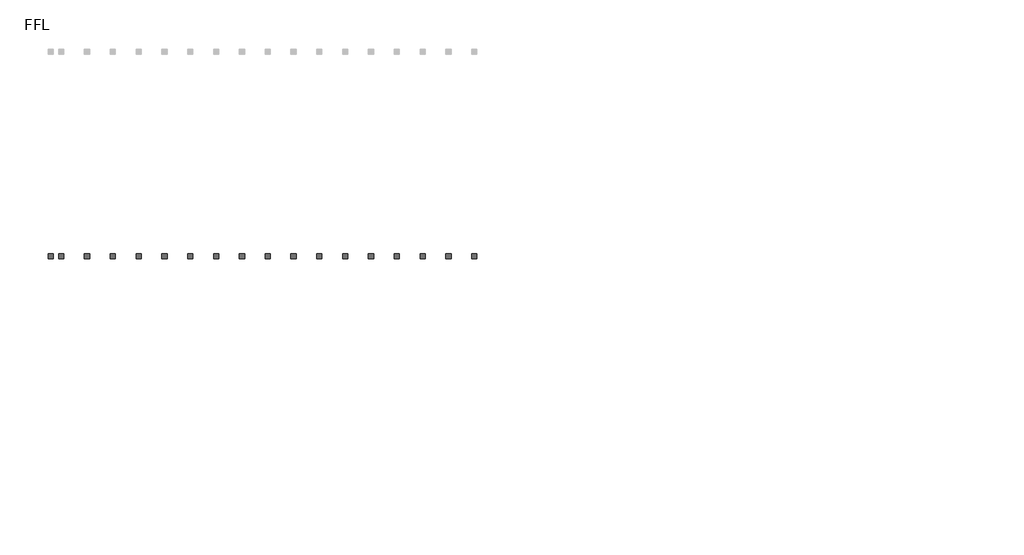
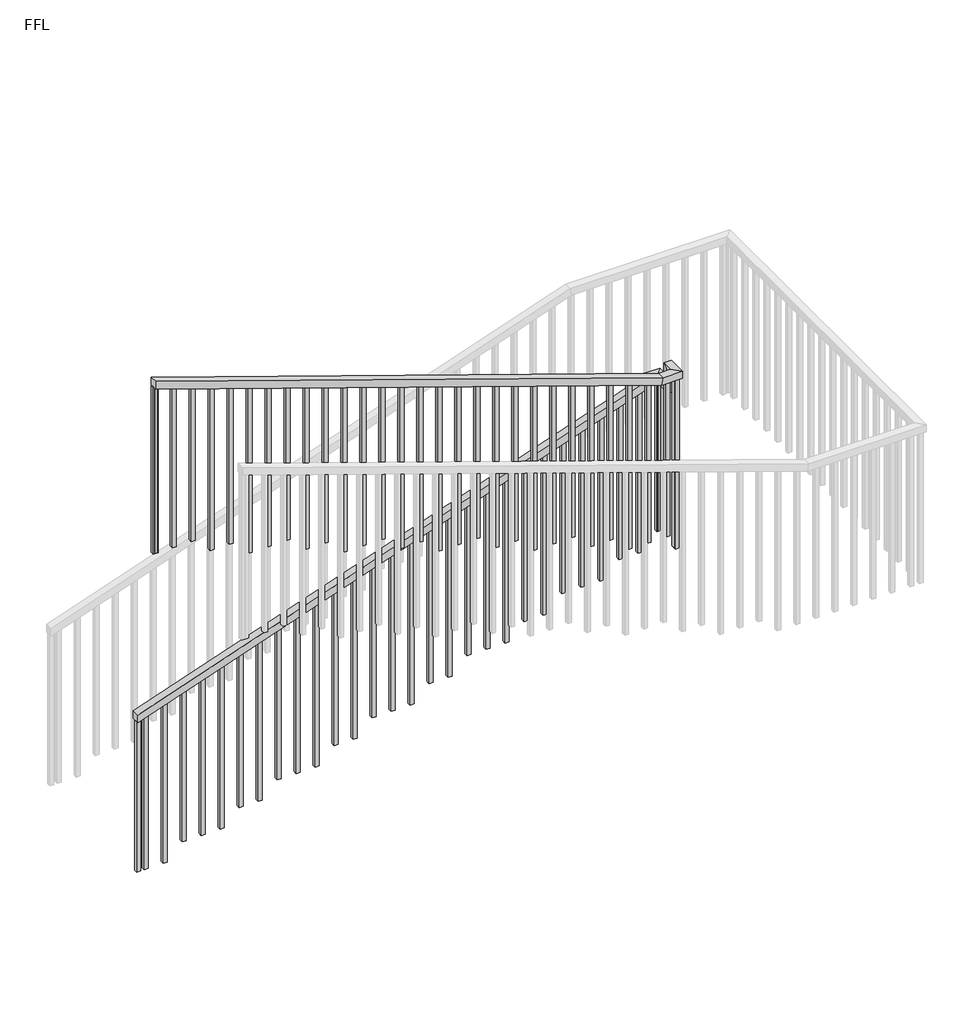
# One storey, part 1 of 2: 1 railing.
"""IFC4 building model written with IfcOpenShell, lengths in millimetres."""

from ifc_helpers import new_model, si_unit, frame, origin, place, context, project, spatial, polyline, outline, extrude, faceted_brep, element, save

model = new_model("IFC4")

# Units and contexts
model_context = context("Model", 3, world=origin())
ifc_project = project(units=[si_unit("LENGTHUNIT", "METRE", prefix="MILLI")], contexts=[model_context])

# Site, building, storey
site = spatial("IfcSite", under=ifc_project)
building = spatial("IfcBuilding", under=site)
storey = spatial("IfcBuildingStorey", under=building, Name="FFL", Elevation=3000.0)

# Railing
placement = place(None, origin())
element("IfcRailing", 1, ObjectType="1100mm", at=placement, inside=storey, context=model_context, shape_type="SolidModel", body=[
    faceted_brep([(-40149.9681829, 16845.7531621, 4656.2088216), (-40149.9681829, 16845.7531621, 4603.3636913), (-40149.9681829, 16795.7531621, 4603.3636913), (-40149.9681829, 16795.7531621, 4656.2088216), (-36808.2681829, 16845.7531621, 5799.4566882), (-36758.2681829, 16845.7531621, 5763.7173404), (-36758.2681829, 16795.7531621, 5763.7173404), (-36808.2681829, 16795.7531621, 5799.4566882), (-36808.2681829, 16845.7531621, 5824.9785156), (-36758.2681829, 16845.7531621, 5774.9785156), (-36758.2681829, 16795.7531621, 5774.9785156), (-36808.2681829, 16795.7531621, 5824.9785156), (-36683.2681829, 16845.7531621, 5824.9785156), (-36683.2681829, 16845.7531621, 5774.9785156), (-36733.2681829, 16795.7531621, 5774.9785156), (-36733.2681829, 16795.7531621, 5824.9785156), (-36683.2681829, 16720.7531621, 5824.9785156), (-36683.2681829, 16720.7531621, 5774.9785156), (-36733.2681829, 16720.7531621, 5774.9785156), (-36733.2681829, 16720.7531621, 5824.9785156), (-36683.2681829, 16717.5531621, 5824.9785156), (-36683.2681829, 16667.5531621, 5774.9785156), (-36733.2681829, 16667.5531621, 5774.9785156), (-36733.2681829, 16717.5531621, 5824.9785156), (-36683.2681829, 16717.5531621, 5956.7521335), (-36683.2681829, 16667.5531621, 5906.7521335), (-36733.2681829, 16667.5531621, 5906.7521335), (-36733.2681829, 16717.5531621, 5956.7521335), (-36683.2681829, 16592.5531621, 5956.7521335), (-36683.2681829, 16592.5531621, 5906.7521335), (-36733.2681829, 16642.5531621, 5906.7521335), (-36733.2681829, 16642.5531621, 5956.7521335), (-36808.2681829, 16592.5531621, 5956.7521335), (-36816.5844651, 16592.5531621, 5906.7521335), (-36816.5844651, 16642.5531621, 5906.7521335), (-36808.2681829, 16642.5531621, 5956.7521335), (-40149.9681829, 16592.5531621, 7100.0), (-40149.9681829, 16642.5531621, 7100.0), (-40149.9681829, 16642.5531621, 7047.1548697), (-40149.9681829, 16592.5531621, 7047.1548697)], [[[0, 1, 2, 3]], [[1, 0, 4, 5]], [[2, 1, 5, 6]], [[3, 2, 6, 7]], [[0, 3, 7, 4]], [[5, 4, 8, 9]], [[6, 5, 9, 10]], [[7, 6, 10, 11]], [[4, 7, 11, 8]], [[9, 8, 12, 13]], [[10, 9, 13, 14]], [[11, 10, 14, 15]], [[8, 11, 15, 12]], [[13, 12, 16, 17]], [[14, 13, 17, 18]], [[15, 14, 18, 19]], [[12, 15, 19, 16]], [[17, 16, 20, 21]], [[18, 17, 21, 22]], [[19, 18, 22, 23]], [[16, 19, 23, 20]], [[21, 20, 24, 25]], [[22, 21, 25, 26]], [[23, 22, 26, 27]], [[20, 23, 27, 24]], [[25, 24, 28, 29]], [[26, 25, 29, 30]], [[27, 26, 30, 31]], [[24, 27, 31, 28]], [[29, 28, 32, 33]], [[30, 29, 33, 34]], [[31, 30, 34, 35]], [[28, 31, 35, 32]], [[36, 37, 38, 39]], [[33, 32, 36, 39]], [[34, 33, 39, 38]], [[35, 34, 38, 37]], [[32, 35, 37, 36]]]),
    extrude(outline(polyline([(5893.7482096, -40133.2681829), (7041.4415384, -40133.2681829), (7049.9944296, -40158.2681829), (5893.7482096, -40158.2681829), (5893.7482096, -40133.2681829)])), frame((0.0, 16605.0531621, 0.0), z_axis=(0.0, 1.0, 0.0), x_axis=(0.0, 0.0, 1.0)), (0.0, 0.0, 1.0), 25.0),
    extrude(outline(polyline([(5893.7482096, -40008.2681829), (6998.6770822, -40008.2681829), (7007.2299734, -40033.2681829), (5893.7482096, -40033.2681829), (5893.7482096, -40008.2681829)])), frame((0.0, 16605.0531621, 0.0), z_axis=(0.0, 1.0, 0.0), x_axis=(0.0, 0.0, 1.0)), (0.0, 0.0, 1.0), 25.0),
    extrude(outline(polyline([(5893.7482096, -39883.2681829), (6955.9126259, -39883.2681829), (6964.4655172, -39908.2681829), (5893.7482096, -39908.2681829), (5893.7482096, -39883.2681829)])), frame((0.0, 16605.0531621, 0.0), z_axis=(0.0, 1.0, 0.0), x_axis=(0.0, 0.0, 1.0)), (0.0, 0.0, 1.0), 25.0),
    extrude(outline(polyline([(5787.4964193, -39758.2681829), (6913.1481697, -39758.2681829), (6921.701061, -39783.2681829), (5787.4964193, -39783.2681829), (5787.4964193, -39758.2681829)])), frame((0.0, 16605.0531621, 0.0), z_axis=(0.0, 1.0, 0.0), x_axis=(0.0, 0.0, 1.0)), (0.0, 0.0, 1.0), 25.0),
    extrude(outline(polyline([(5787.4964193, -39633.2681829), (6870.3837135, -39633.2681829), (6878.9366048, -39658.2681829), (5787.4964193, -39658.2681829), (5787.4964193, -39633.2681829)])), frame((0.0, 16605.0531621, 0.0), z_axis=(0.0, 1.0, 0.0), x_axis=(0.0, 0.0, 1.0)), (0.0, 0.0, 1.0), 25.0),
    extrude(outline(polyline([(5681.2446289, -39508.2681829), (6827.6192573, -39508.2681829), (6836.1721486, -39533.2681829), (5681.2446289, -39533.2681829), (5681.2446289, -39508.2681829)])), frame((0.0, 16605.0531621, 0.0), z_axis=(0.0, 1.0, 0.0), x_axis=(0.0, 0.0, 1.0)), (0.0, 0.0, 1.0), 25.0),
    extrude(outline(polyline([(5681.2446289, -39383.2681829), (6784.8548011, -39383.2681829), (6793.4076923, -39408.2681829), (5681.2446289, -39408.2681829), (5681.2446289, -39383.2681829)])), frame((0.0, 16605.0531621, 0.0), z_axis=(0.0, 1.0, 0.0), x_axis=(0.0, 0.0, 1.0)), (0.0, 0.0, 1.0), 25.0),
    extrude(outline(polyline([(5681.2446289, -39258.2681829), (6742.0903449, -39258.2681829), (6750.6432361, -39283.2681829), (5681.2446289, -39283.2681829), (5681.2446289, -39258.2681829)])), frame((0.0, 16605.0531621, 0.0), z_axis=(0.0, 1.0, 0.0), x_axis=(0.0, 0.0, 1.0)), (0.0, 0.0, 1.0), 25.0),
    extrude(outline(polyline([(5574.9928385, -39133.2681829), (6699.3258887, -39133.2681829), (6707.8787799, -39158.2681829), (5574.9928385, -39158.2681829), (5574.9928385, -39133.2681829)])), frame((0.0, 16605.0531621, 0.0), z_axis=(0.0, 1.0, 0.0), x_axis=(0.0, 0.0, 1.0)), (0.0, 0.0, 1.0), 25.0),
    extrude(outline(polyline([(5574.9928385, -39008.2681829), (6656.5614325, -39008.2681829), (6665.1143237, -39033.2681829), (5574.9928385, -39033.2681829), (5574.9928385, -39008.2681829)])), frame((0.0, 16605.0531621, 0.0), z_axis=(0.0, 1.0, 0.0), x_axis=(0.0, 0.0, 1.0)), (0.0, 0.0, 1.0), 25.0),
    extrude(outline(polyline([(5468.7410482, -38883.2681829), (6613.7969763, -38883.2681829), (6622.3498675, -38908.2681829), (5468.7410482, -38908.2681829), (5468.7410482, -38883.2681829)])), frame((0.0, 16605.0531621, 0.0), z_axis=(0.0, 1.0, 0.0), x_axis=(0.0, 0.0, 1.0)), (0.0, 0.0, 1.0), 25.0),
    extrude(outline(polyline([(5468.7410482, -38758.2681829), (6571.0325201, -38758.2681829), (6579.5854113, -38783.2681829), (5468.7410482, -38783.2681829), (5468.7410482, -38758.2681829)])), frame((0.0, 16605.0531621, 0.0), z_axis=(0.0, 1.0, 0.0), x_axis=(0.0, 0.0, 1.0)), (0.0, 0.0, 1.0), 25.0),
    extrude(outline(polyline([(5468.7410482, -38633.2681829), (6528.2680638, -38633.2681829), (6536.8209551, -38658.2681829), (5468.7410482, -38658.2681829), (5468.7410482, -38633.2681829)])), frame((0.0, 16605.0531621, 0.0), z_axis=(0.0, 1.0, 0.0), x_axis=(0.0, 0.0, 1.0)), (0.0, 0.0, 1.0), 25.0),
    extrude(outline(polyline([(5362.4892578, -38508.2681829), (6485.5036076, -38508.2681829), (6494.0564989, -38533.2681829), (5362.4892578, -38533.2681829), (5362.4892578, -38508.2681829)])), frame((0.0, 16605.0531621, 0.0), z_axis=(0.0, 1.0, 0.0), x_axis=(0.0, 0.0, 1.0)), (0.0, 0.0, 1.0), 25.0),
    extrude(outline(polyline([(5362.4892578, -38383.2681829), (6442.7391514, -38383.2681829), (6451.2920427, -38408.2681829), (5362.4892578, -38408.2681829), (5362.4892578, -38383.2681829)])), frame((0.0, 16605.0531621, 0.0), z_axis=(0.0, 1.0, 0.0), x_axis=(0.0, 0.0, 1.0)), (0.0, 0.0, 1.0), 25.0),
    extrude(outline(polyline([(5256.2374674, -38258.2681829), (6399.9746952, -38258.2681829), (6408.5275865, -38283.2681829), (5256.2374674, -38283.2681829), (5256.2374674, -38258.2681829)])), frame((0.0, 16605.0531621, 0.0), z_axis=(0.0, 1.0, 0.0), x_axis=(0.0, 0.0, 1.0)), (0.0, 0.0, 1.0), 25.0),
    extrude(outline(polyline([(5256.2374674, -38133.2681829), (6357.210239, -38133.2681829), (6365.7631302, -38158.2681829), (5256.2374674, -38158.2681829), (5256.2374674, -38133.2681829)])), frame((0.0, 16605.0531621, 0.0), z_axis=(0.0, 1.0, 0.0), x_axis=(0.0, 0.0, 1.0)), (0.0, 0.0, 1.0), 25.0),
    extrude(outline(polyline([(5256.2374674, -38008.2681829), (6314.4457828, -38008.2681829), (6322.998674, -38033.2681829), (5256.2374674, -38033.2681829), (5256.2374674, -38008.2681829)])), frame((0.0, 16605.0531621, 0.0), z_axis=(0.0, 1.0, 0.0), x_axis=(0.0, 0.0, 1.0)), (0.0, 0.0, 1.0), 25.0),
    extrude(outline(polyline([(5149.9856771, -37883.2681829), (6271.6813266, -37883.2681829), (6280.2342178, -37908.2681829), (5149.9856771, -37908.2681829), (5149.9856771, -37883.2681829)])), frame((0.0, 16605.0531621, 0.0), z_axis=(0.0, 1.0, 0.0), x_axis=(0.0, 0.0, 1.0)), (0.0, 0.0, 1.0), 25.0),
    extrude(outline(polyline([(5149.9856771, -37758.2681829), (6228.9168704, -37758.2681829), (6237.4697616, -37783.2681829), (5149.9856771, -37783.2681829), (5149.9856771, -37758.2681829)])), frame((0.0, 16605.0531621, 0.0), z_axis=(0.0, 1.0, 0.0), x_axis=(0.0, 0.0, 1.0)), (0.0, 0.0, 1.0), 25.0),
    extrude(outline(polyline([(5043.7338867, -37633.2681829), (6186.1524142, -37633.2681829), (6194.7053054, -37658.2681829), (5043.7338867, -37658.2681829), (5043.7338867, -37633.2681829)])), frame((0.0, 16605.0531621, 0.0), z_axis=(0.0, 1.0, 0.0), x_axis=(0.0, 0.0, 1.0)), (0.0, 0.0, 1.0), 25.0),
    extrude(outline(polyline([(5043.7338867, -37508.2681829), (6143.387958, -37508.2681829), (6151.9408492, -37533.2681829), (5043.7338867, -37533.2681829), (5043.7338867, -37508.2681829)])), frame((0.0, 16605.0531621, 0.0), z_axis=(0.0, 1.0, 0.0), x_axis=(0.0, 0.0, 1.0)), (0.0, 0.0, 1.0), 25.0),
    extrude(outline(polyline([(5043.7338867, -37383.2681829), (6100.6235017, -37383.2681829), (6109.176393, -37408.2681829), (5043.7338867, -37408.2681829), (5043.7338867, -37383.2681829)])), frame((0.0, 16605.0531621, 0.0), z_axis=(0.0, 1.0, 0.0), x_axis=(0.0, 0.0, 1.0)), (0.0, 0.0, 1.0), 25.0),
    extrude(outline(polyline([(4937.4820964, -37258.2681829), (6057.8590455, -37258.2681829), (6066.4119368, -37283.2681829), (4937.4820964, -37283.2681829), (4937.4820964, -37258.2681829)])), frame((0.0, 16605.0531621, 0.0), z_axis=(0.0, 1.0, 0.0), x_axis=(0.0, 0.0, 1.0)), (0.0, 0.0, 1.0), 25.0),
    extrude(outline(polyline([(4937.4820964, -37133.2681829), (6015.0945893, -37133.2681829), (6023.6474806, -37158.2681829), (4937.4820964, -37158.2681829), (4937.4820964, -37133.2681829)])), frame((0.0, 16605.0531621, 0.0), z_axis=(0.0, 1.0, 0.0), x_axis=(0.0, 0.0, 1.0)), (0.0, 0.0, 1.0), 25.0),
    extrude(outline(polyline([(4831.230306, -37008.2681829), (5972.3301331, -37008.2681829), (5980.8830244, -37033.2681829), (4831.230306, -37033.2681829), (4831.230306, -37008.2681829)])), frame((0.0, 16605.0531621, 0.0), z_axis=(0.0, 1.0, 0.0), x_axis=(0.0, 0.0, 1.0)), (0.0, 0.0, 1.0), 25.0),
    extrude(outline(polyline([(4831.230306, -36883.2681829), (5929.5656769, -36883.2681829), (5938.1185681, -36908.2681829), (4831.230306, -36908.2681829), (4831.230306, -36883.2681829)])), frame((0.0, 16605.0531621, 0.0), z_axis=(0.0, 1.0, 0.0), x_axis=(0.0, 0.0, 1.0)), (0.0, 0.0, 1.0), 25.0),
    extrude(outline(polyline([(-36758.2681829, 16630.0531621), (-36758.2681829, 16605.0531621), (-36783.2681829, 16605.0531621), (-36783.2681829, 16630.0531621), (-36758.2681829, 16630.0531621)])), frame((0.0, 0.0, 4831.230306), z_axis=(0.0, 0.0, 1.0), x_axis=(1.0, 0.0, 0.0)), (0.0, 0.0, 1.0), 1075.5218275),
    extrude(outline(polyline([(-36720.7681829, 16645.7531621), (-36695.7681829, 16645.7531621), (-36695.7681829, 16620.7531621), (-36720.7681829, 16620.7531621), (-36720.7681829, 16645.7531621)])), frame((0.0, 0.0, 4724.9785156), z_axis=(0.0, 0.0, 1.0), x_axis=(1.0, 0.0, 0.0)), (0.0, 0.0, 1.0), 1181.7736178),
    extrude(outline(polyline([(-36720.7681829, 16770.7531621), (-36695.7681829, 16770.7531621), (-36695.7681829, 16745.7531621), (-36720.7681829, 16745.7531621), (-36720.7681829, 16770.7531621)])), frame((0.0, 0.0, 4724.9785156), z_axis=(0.0, 0.0, 1.0), x_axis=(1.0, 0.0, 0.0)), (0.0, 0.0, 1.0), 1050.0),
    extrude(outline(polyline([(-36724.9681829, 16808.2531621), (-36724.9681829, 16833.2531621), (-36699.9681829, 16833.2531621), (-36699.9681829, 16808.2531621), (-36724.9681829, 16808.2531621)])), frame((0.0, 0.0, 4724.9785156), z_axis=(0.0, 0.0, 1.0), x_axis=(1.0, 0.0, 0.0)), (0.0, 0.0, 1.0), 1050.0),
    extrude(outline(polyline([(5732.3453353, -36849.9681829), (4618.7267253, -36849.9681829), (4618.7267253, -36824.9681829), (5740.8982265, -36824.9681829), (5732.3453353, -36849.9681829)])), frame((0.0, 16808.2531621, 0.0), z_axis=(0.0, 1.0, 0.0), x_axis=(0.0, 0.0, 1.0)), (0.0, 0.0, 1.0), 25.0),
    extrude(outline(polyline([(5689.5808791, -36974.9681829), (4618.7267253, -36974.9681829), (4618.7267253, -36949.9681829), (5698.1337703, -36949.9681829), (5689.5808791, -36974.9681829)])), frame((0.0, 16808.2531621, 0.0), z_axis=(0.0, 1.0, 0.0), x_axis=(0.0, 0.0, 1.0)), (0.0, 0.0, 1.0), 25.0),
    extrude(outline(polyline([(5646.8164229, -37099.9681829), (4512.4749349, -37099.9681829), (4512.4749349, -37074.9681829), (5655.3693141, -37074.9681829), (5646.8164229, -37099.9681829)])), frame((0.0, 16808.2531621, 0.0), z_axis=(0.0, 1.0, 0.0), x_axis=(0.0, 0.0, 1.0)), (0.0, 0.0, 1.0), 25.0),
    extrude(outline(polyline([(5604.0519667, -37224.9681829), (4512.4749349, -37224.9681829), (4512.4749349, -37199.9681829), (5612.6048579, -37199.9681829), (5604.0519667, -37224.9681829)])), frame((0.0, 16808.2531621, 0.0), z_axis=(0.0, 1.0, 0.0), x_axis=(0.0, 0.0, 1.0)), (0.0, 0.0, 1.0), 25.0),
    extrude(outline(polyline([(5561.2875104, -37349.9681829), (4512.4749349, -37349.9681829), (4512.4749349, -37324.9681829), (5569.8404017, -37324.9681829), (5561.2875104, -37349.9681829)])), frame((0.0, 16808.2531621, 0.0), z_axis=(0.0, 1.0, 0.0), x_axis=(0.0, 0.0, 1.0)), (0.0, 0.0, 1.0), 25.0),
    extrude(outline(polyline([(5518.5230542, -37474.9681829), (4406.2231445, -37474.9681829), (4406.2231445, -37449.9681829), (5527.0759455, -37449.9681829), (5518.5230542, -37474.9681829)])), frame((0.0, 16808.2531621, 0.0), z_axis=(0.0, 1.0, 0.0), x_axis=(0.0, 0.0, 1.0)), (0.0, 0.0, 1.0), 25.0),
    extrude(outline(polyline([(5475.758598, -37599.9681829), (4406.2231445, -37599.9681829), (4406.2231445, -37574.9681829), (5484.3114893, -37574.9681829), (5475.758598, -37599.9681829)])), frame((0.0, 16808.2531621, 0.0), z_axis=(0.0, 1.0, 0.0), x_axis=(0.0, 0.0, 1.0)), (0.0, 0.0, 1.0), 25.0),
    extrude(outline(polyline([(5432.9941418, -37724.9681829), (4299.9713542, -37724.9681829), (4299.9713542, -37699.9681829), (5441.5470331, -37699.9681829), (5432.9941418, -37724.9681829)])), frame((0.0, 16808.2531621, 0.0), z_axis=(0.0, 1.0, 0.0), x_axis=(0.0, 0.0, 1.0)), (0.0, 0.0, 1.0), 25.0),
    extrude(outline(polyline([(5390.2296856, -37849.9681829), (4299.9713542, -37849.9681829), (4299.9713542, -37824.9681829), (5398.7825768, -37824.9681829), (5390.2296856, -37849.9681829)])), frame((0.0, 16808.2531621, 0.0), z_axis=(0.0, 1.0, 0.0), x_axis=(0.0, 0.0, 1.0)), (0.0, 0.0, 1.0), 25.0),
    extrude(outline(polyline([(5347.4652294, -37974.9681829), (4299.9713542, -37974.9681829), (4299.9713542, -37949.9681829), (5356.0181206, -37949.9681829), (5347.4652294, -37974.9681829)])), frame((0.0, 16808.2531621, 0.0), z_axis=(0.0, 1.0, 0.0), x_axis=(0.0, 0.0, 1.0)), (0.0, 0.0, 1.0), 25.0),
    extrude(outline(polyline([(5304.7007732, -38099.9681829), (4193.7195638, -38099.9681829), (4193.7195638, -38074.9681829), (5313.2536644, -38074.9681829), (5304.7007732, -38099.9681829)])), frame((0.0, 16808.2531621, 0.0), z_axis=(0.0, 1.0, 0.0), x_axis=(0.0, 0.0, 1.0)), (0.0, 0.0, 1.0), 25.0),
    extrude(outline(polyline([(5261.936317, -38224.9681829), (4193.7195638, -38224.9681829), (4193.7195638, -38199.9681829), (5270.4892082, -38199.9681829), (5261.936317, -38224.9681829)])), frame((0.0, 16808.2531621, 0.0), z_axis=(0.0, 1.0, 0.0), x_axis=(0.0, 0.0, 1.0)), (0.0, 0.0, 1.0), 25.0),
    extrude(outline(polyline([(5219.1718608, -38349.9681829), (4087.4677734, -38349.9681829), (4087.4677734, -38324.9681829), (5227.724752, -38324.9681829), (5219.1718608, -38349.9681829)])), frame((0.0, 16808.2531621, 0.0), z_axis=(0.0, 1.0, 0.0), x_axis=(0.0, 0.0, 1.0)), (0.0, 0.0, 1.0), 25.0),
    extrude(outline(polyline([(5176.4074046, -38474.9681829), (4087.4677734, -38474.9681829), (4087.4677734, -38449.9681829), (5184.9602958, -38449.9681829), (5176.4074046, -38474.9681829)])), frame((0.0, 16808.2531621, 0.0), z_axis=(0.0, 1.0, 0.0), x_axis=(0.0, 0.0, 1.0)), (0.0, 0.0, 1.0), 25.0),
    extrude(outline(polyline([(5133.6429483, -38599.9681829), (4087.4677734, -38599.9681829), (4087.4677734, -38574.9681829), (5142.1958396, -38574.9681829), (5133.6429483, -38599.9681829)])), frame((0.0, 16808.2531621, 0.0), z_axis=(0.0, 1.0, 0.0), x_axis=(0.0, 0.0, 1.0)), (0.0, 0.0, 1.0), 25.0),
    extrude(outline(polyline([(5090.8784921, -38724.9681829), (3981.2159831, -38724.9681829), (3981.2159831, -38699.9681829), (5099.4313834, -38699.9681829), (5090.8784921, -38724.9681829)])), frame((0.0, 16808.2531621, 0.0), z_axis=(0.0, 1.0, 0.0), x_axis=(0.0, 0.0, 1.0)), (0.0, 0.0, 1.0), 25.0),
    extrude(outline(polyline([(5048.1140359, -38849.9681829), (3981.2159831, -38849.9681829), (3981.2159831, -38824.9681829), (5056.6669272, -38824.9681829), (5048.1140359, -38849.9681829)])), frame((0.0, 16808.2531621, 0.0), z_axis=(0.0, 1.0, 0.0), x_axis=(0.0, 0.0, 1.0)), (0.0, 0.0, 1.0), 25.0),
    extrude(outline(polyline([(5005.3495797, -38974.9681829), (3874.9641927, -38974.9681829), (3874.9641927, -38949.9681829), (5013.902471, -38949.9681829), (5005.3495797, -38974.9681829)])), frame((0.0, 16808.2531621, 0.0), z_axis=(0.0, 1.0, 0.0), x_axis=(0.0, 0.0, 1.0)), (0.0, 0.0, 1.0), 25.0),
    extrude(outline(polyline([(4962.5851235, -39099.9681829), (3874.9641927, -39099.9681829), (3874.9641927, -39074.9681829), (4971.1380147, -39074.9681829), (4962.5851235, -39099.9681829)])), frame((0.0, 16808.2531621, 0.0), z_axis=(0.0, 1.0, 0.0), x_axis=(0.0, 0.0, 1.0)), (0.0, 0.0, 1.0), 25.0),
    extrude(outline(polyline([(4919.8206673, -39224.9681829), (3874.9641927, -39224.9681829), (3874.9641927, -39199.9681829), (4928.3735585, -39199.9681829), (4919.8206673, -39224.9681829)])), frame((0.0, 16808.2531621, 0.0), z_axis=(0.0, 1.0, 0.0), x_axis=(0.0, 0.0, 1.0)), (0.0, 0.0, 1.0), 25.0),
    extrude(outline(polyline([(4877.0562111, -39349.9681829), (3768.7124023, -39349.9681829), (3768.7124023, -39324.9681829), (4885.6091023, -39324.9681829), (4877.0562111, -39349.9681829)])), frame((0.0, 16808.2531621, 0.0), z_axis=(0.0, 1.0, 0.0), x_axis=(0.0, 0.0, 1.0)), (0.0, 0.0, 1.0), 25.0),
    extrude(outline(polyline([(4834.2917549, -39474.9681829), (3768.7124023, -39474.9681829), (3768.7124023, -39449.9681829), (4842.8446461, -39449.9681829), (4834.2917549, -39474.9681829)])), frame((0.0, 16808.2531621, 0.0), z_axis=(0.0, 1.0, 0.0), x_axis=(0.0, 0.0, 1.0)), (0.0, 0.0, 1.0), 25.0),
    extrude(outline(polyline([(4791.5272987, -39599.9681829), (3662.460612, -39599.9681829), (3662.460612, -39574.9681829), (4800.0801899, -39574.9681829), (4791.5272987, -39599.9681829)])), frame((0.0, 16808.2531621, 0.0), z_axis=(0.0, 1.0, 0.0), x_axis=(0.0, 0.0, 1.0)), (0.0, 0.0, 1.0), 25.0),
    extrude(outline(polyline([(4748.7628424, -39724.9681829), (3662.460612, -39724.9681829), (3662.460612, -39699.9681829), (4757.3157337, -39699.9681829), (4748.7628424, -39724.9681829)])), frame((0.0, 16808.2531621, 0.0), z_axis=(0.0, 1.0, 0.0), x_axis=(0.0, 0.0, 1.0)), (0.0, 0.0, 1.0), 25.0),
    extrude(outline(polyline([(4705.9983862, -39849.9681829), (3662.460612, -39849.9681829), (3662.460612, -39824.9681829), (4714.5512775, -39824.9681829), (4705.9983862, -39849.9681829)])), frame((0.0, 16808.2531621, 0.0), z_axis=(0.0, 1.0, 0.0), x_axis=(0.0, 0.0, 1.0)), (0.0, 0.0, 1.0), 25.0),
    extrude(outline(polyline([(4663.23393, -39974.9681829), (3556.2088216, -39974.9681829), (3556.2088216, -39949.9681829), (4671.7868213, -39949.9681829), (4663.23393, -39974.9681829)])), frame((0.0, 16808.2531621, 0.0), z_axis=(0.0, 1.0, 0.0), x_axis=(0.0, 0.0, 1.0)), (0.0, 0.0, 1.0), 25.0),
    extrude(outline(polyline([(4620.4694738, -40099.9681829), (3556.2088216, -40099.9681829), (3556.2088216, -40074.9681829), (4629.0223651, -40074.9681829), (4620.4694738, -40099.9681829)])), frame((0.0, 16808.2531621, 0.0), z_axis=(0.0, 1.0, 0.0), x_axis=(0.0, 0.0, 1.0)), (0.0, 0.0, 1.0), 25.0),
    extrude(outline(polyline([(-36720.7681829, 16630.0531621), (-36695.7681829, 16630.0531621), (-36695.7681829, 16605.0531621), (-36720.7681829, 16605.0531621), (-36720.7681829, 16630.0531621)])), frame((0.0, 0.0, 4724.9785156), z_axis=(0.0, 0.0, 1.0), x_axis=(1.0, 0.0, 0.0)), (0.0, 0.0, 1.0), 1181.7736178),
    extrude(outline(polyline([(-36720.7681829, 16808.2531621), (-36720.7681829, 16833.2531621), (-36695.7681829, 16833.2531621), (-36695.7681829, 16808.2531621), (-36720.7681829, 16808.2531621)])), frame((0.0, 0.0, 4724.9785156), z_axis=(0.0, 0.0, 1.0), x_axis=(1.0, 0.0, 0.0)), (0.0, 0.0, 1.0), 1050.0),
    extrude(outline(polyline([(5893.7482096, -40124.9681829), (7038.6019785, -40124.9681829), (7047.1548697, -40149.9681829), (5893.7482096, -40149.9681829), (5893.7482096, -40124.9681829)])), frame((0.0, 16605.0531621, 0.0), z_axis=(0.0, 1.0, 0.0), x_axis=(0.0, 0.0, 1.0)), (0.0, 0.0, 1.0), 25.0),
    extrude(outline(polyline([(4603.3636913, -40149.9681829), (3556.2088216, -40149.9681829), (3556.2088216, -40124.9681829), (4611.9165826, -40124.9681829), (4603.3636913, -40149.9681829)])), frame((0.0, 16808.2531621, 0.0), z_axis=(0.0, 1.0, 0.0), x_axis=(0.0, 0.0, 1.0)), (0.0, 0.0, 1.0), 25.0),
])

save(model, "model.ifc")

# Revit data of these elements
# Type "1100mm"
#   built-in parameter 1008612 = 0.019685 (stored number, unit not read)
#   built-in parameter 1008611 = 0.019685 (stored number, unit not read)
#   built-in parameter 1008609 = 0.902231 (stored number, unit not read)
#   built-in parameter 1008604 = 0.19685 (stored number, unit not read)
#   built-in parameter 1008603 = 0.164042 (stored number, unit not read)
#   Railing Height = 3' - 7.30709"
#   built-in parameter 1008630 = 2
#   built-in parameter 1008610 = 2
#   built-in parameter 1008608 = 1
#   built-in parameter 1008618 = Baluster_Square : 25mm
# Element 1 (IfcRailing, "1100mm")
#   Phase Created = New Construction
